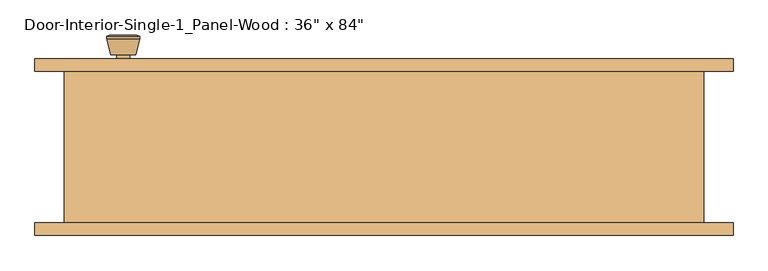
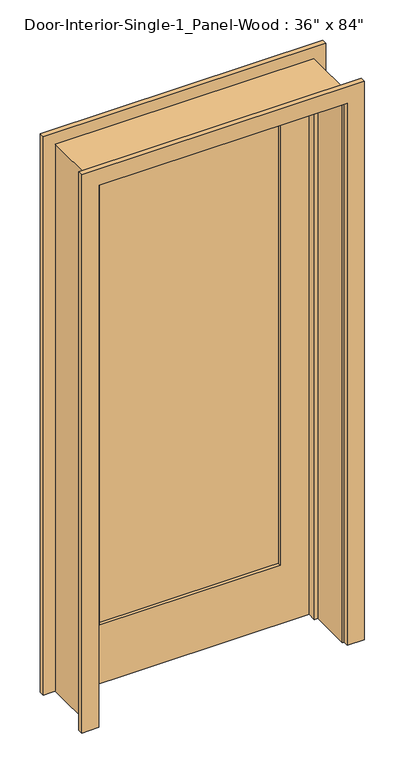
"""IFC4 building model written with IfcOpenShell, lengths in millimetres: door geometry."""

from ifc_helpers import new_model, si_unit, point, frame, frame_2d, origin, place, context, project, spatial, polyline, circle_curve, trimmed, segment, composite_curve, outline, extrude, faceted_brep, source, transform, mapped, element, save
from ifc_brep_helpers import plane_surface, cylinder_surface, revolved_surface, advanced_brep


def door_3b97b8e7(model_context):
    return source(origin(), model_context, "Body", "SolidModel", [
        advanced_brep(
        [(-393.7, 70.2, 914.4), (-383.7, 70.2, 914.4), (-403.7, 70.2, 914.4), (-373.2241324, 21.2, 914.4), (-393.7, 21.2, 914.4), (-414.1758676, 21.2, 914.4), (-368.7, 23.0278681, 914.4), (-418.7, 23.0278681, 914.4), (-368.7, 26.4915463, 914.4), (-418.7, 26.4915463, 914.4), (-375.063764, 51.2, 914.4), (-412.336236, 51.2, 914.4), (-383.7, 51.2, 914.4), (-403.7, 51.2, 914.4)],
        [
            (0, 1),
            (1, 2, circle_curve(frame((-393.7, 70.2, 914.4), z_axis=(0.0, 1.0, 0.0), x_axis=(-1.0, 0.0, 0.0)), 10.0)),
            (2, 0),
            (2, 1, circle_curve(frame((-393.7, 70.2, 914.4), z_axis=(0.0, 1.0, 0.0), x_axis=(-1.0, 0.0, 0.0)), 10.0)),
            (3, 4),
            (4, 5),
            (5, 3, circle_curve(frame((-393.7, 21.2, 914.4), z_axis=(0.0, -1.0, 0.0), x_axis=(-1.0, 0.0, 0.0)), 20.4758676)),
            (3, 5, circle_curve(frame((-393.7, 21.2, 914.4), z_axis=(0.0, -1.0, 0.0), x_axis=(-1.0, 0.0, 0.0)), 20.4758676)),
            (6, 3),
            (5, 7),
            (7, 6, circle_curve(frame((-393.7, 23.0278681, 914.4), z_axis=(0.0, -1.0, 0.0), x_axis=(-1.0, 0.0, 0.0)), 25.0)),
            (6, 7, circle_curve(frame((-393.7, 23.0278681, 914.4), z_axis=(0.0, -1.0, 0.0), x_axis=(-1.0, 0.0, 0.0)), 25.0)),
            (8, 6),
            (7, 9),
            (9, 8, circle_curve(frame((-393.7, 26.4915463, 914.4), z_axis=(0.0, -1.0, 0.0), x_axis=(-1.0, 0.0, 0.0)), 25.0)),
            (8, 9, circle_curve(frame((-393.7, 26.4915463, 914.4), z_axis=(0.0, -1.0, 0.0), x_axis=(-1.0, 0.0, 0.0)), 25.0)),
            (10, 8),
            (9, 11),
            (11, 10, circle_curve(frame((-393.7, 51.2, 914.4), z_axis=(0.0, -1.0, 0.0), x_axis=(-1.0, 0.0, 0.0)), 18.636236)),
            (10, 11, circle_curve(frame((-393.7, 51.2, 914.4), z_axis=(0.0, -1.0, 0.0), x_axis=(-1.0, 0.0, 0.0)), 18.636236)),
            (12, 10),
            (11, 13),
            (13, 12, circle_curve(frame((-393.7, 51.2, 914.4), z_axis=(0.0, -1.0, 0.0), x_axis=(-1.0, 0.0, 0.0)), 10.0)),
            (12, 13, circle_curve(frame((-393.7, 51.2, 914.4), z_axis=(0.0, -1.0, 0.0), x_axis=(-1.0, 0.0, 0.0)), 10.0)),
            (1, 12),
            (13, 2),
        ],
        [
            plane_surface(frame((-393.7, 70.2, 914.4), z_axis=(0.0, 1.0, 0.0), x_axis=(-1.0, 0.0, 0.0))),
            plane_surface(frame((-393.7, 21.2, 914.4), z_axis=(0.0, -1.0, 0.0), x_axis=(-1.0, 0.0, 0.0))),
            revolved_surface(polyline([(-414.1758676, 21.2, 914.4), (-418.7, 23.0278681, 914.4)]), (-393.7, 70.2, 914.4), (0.0, 1.0, 0.0)),
            cylinder_surface(frame((-393.7, 70.2, 914.4), z_axis=(0.0, 1.0, 0.0), x_axis=(-1.0, 0.0, 0.0)), 25.0),
            revolved_surface(polyline([(-418.7, 26.4915463, 914.4), (-412.336236, 51.2, 914.4)]), (-393.7, 70.2, 914.4), (0.0, 1.0, 0.0)),
            plane_surface(frame((-393.7, 51.2, 914.4), z_axis=(0.0, 1.0, 0.0), x_axis=(-1.0, 0.0, 0.0))),
            cylinder_surface(frame((-393.7, 70.2, 914.4), z_axis=(0.0, 1.0, 0.0), x_axis=(-1.0, 0.0, 0.0)), 10.0),
        ],
        [
            (0, [[1, 2, 3]]),
            (0, [[-3, 4, -1]]),
            (1, [[5, 6, 7]]),
            (1, [[-6, -5, 8]]),
            (2, [[9, -7, 10, 11]]),
            (2, [[-10, -8, -9, 12]]),
            (3, [[13, -11, 14, 15]]),
            (3, [[-14, -12, -13, 16]]),
            (4, [[17, -15, 18, 19]]),
            (4, [[-18, -16, -17, 20]]),
            (5, [[21, -19, 22, 23]]),
            (5, [[-22, -20, -21, 24]]),
            (6, [[25, -23, 26, -2]]),
            (6, [[-26, -24, -25, -4]]),
        ],
    ),
        extrude(outline(composite_curve([segment(trimmed(circle_curve(frame_2d((914.4, -393.7)), 30.0), [point((914.4, -423.7))], [point((914.4, -363.7))], False, "CARTESIAN"), True, "CONTINUOUS"), segment(trimmed(circle_curve(frame_2d((914.4, -393.7)), 30.0), [point((914.4, -363.7))], [point((914.4, -423.7))], False, "CARTESIAN"), True, "CONTINUOUS")], self_intersect=False)), frame((0.0, 70.2, 0.0), z_axis=(0.0, 1.0, 0.0), x_axis=(0.0, 0.0, 1.0)), (0.0, 0.0, 1.0), 6.0),
        advanced_brep(
        [(-393.7, 117.125, 914.4), (-403.7, 117.125, 914.4), (-383.7, 117.125, 914.4), (-373.2241324, 166.125, 914.4), (-414.1758676, 166.125, 914.4), (-393.7, 166.125, 914.4), (-368.7, 164.2971319, 914.4), (-418.7, 164.2971319, 914.4), (-368.7, 160.8334537, 914.4), (-418.7, 160.8334537, 914.4), (-375.063764, 136.125, 914.4), (-412.336236, 136.125, 914.4), (-383.7, 136.125, 914.4), (-403.7, 136.125, 914.4)],
        [
            (0, 1),
            (1, 2, circle_curve(frame((-393.7, 117.125, 914.4), z_axis=(0.0, -1.0, 0.0), x_axis=(-1.0, 0.0, 0.0)), 10.0)),
            (2, 0),
            (2, 1, circle_curve(frame((-393.7, 117.125, 914.4), z_axis=(0.0, -1.0, 0.0), x_axis=(-1.0, 0.0, 0.0)), 10.0)),
            (3, 4, circle_curve(frame((-393.7, 166.125, 914.4), z_axis=(0.0, 1.0, 0.0), x_axis=(-1.0, 0.0, 0.0)), 20.4758676)),
            (4, 5),
            (5, 3),
            (4, 3, circle_curve(frame((-393.7, 166.125, 914.4), z_axis=(0.0, 1.0, 0.0), x_axis=(-1.0, 0.0, 0.0)), 20.4758676)),
            (6, 7, circle_curve(frame((-393.7, 164.2971319, 914.4), z_axis=(0.0, 1.0, 0.0), x_axis=(-1.0, 0.0, 0.0)), 25.0)),
            (7, 4),
            (3, 6),
            (7, 6, circle_curve(frame((-393.7, 164.2971319, 914.4), z_axis=(0.0, 1.0, 0.0), x_axis=(-1.0, 0.0, 0.0)), 25.0)),
            (8, 9, circle_curve(frame((-393.7, 160.8334537, 914.4), z_axis=(0.0, 1.0, 0.0), x_axis=(-1.0, 0.0, 0.0)), 25.0)),
            (9, 7),
            (6, 8),
            (9, 8, circle_curve(frame((-393.7, 160.8334537, 914.4), z_axis=(0.0, 1.0, 0.0), x_axis=(-1.0, 0.0, 0.0)), 25.0)),
            (10, 11, circle_curve(frame((-393.7, 136.125, 914.4), z_axis=(0.0, 1.0, 0.0), x_axis=(-1.0, 0.0, 0.0)), 18.636236)),
            (11, 9),
            (8, 10),
            (11, 10, circle_curve(frame((-393.7, 136.125, 914.4), z_axis=(0.0, 1.0, 0.0), x_axis=(-1.0, 0.0, 0.0)), 18.636236)),
            (12, 13, circle_curve(frame((-393.7, 136.125, 914.4), z_axis=(0.0, 1.0, 0.0), x_axis=(-1.0, 0.0, 0.0)), 10.0)),
            (13, 11),
            (10, 12),
            (13, 12, circle_curve(frame((-393.7, 136.125, 914.4), z_axis=(0.0, 1.0, 0.0), x_axis=(-1.0, 0.0, 0.0)), 10.0)),
            (1, 13),
            (12, 2),
        ],
        [
            plane_surface(frame((-393.7, 117.125, 914.4), z_axis=(0.0, -1.0, 0.0), x_axis=(-1.0, 0.0, 0.0))),
            plane_surface(frame((-393.7, 166.125, 914.4), z_axis=(0.0, 1.0, 0.0), x_axis=(-1.0, 0.0, 0.0))),
            revolved_surface(polyline([(-414.1758676, 166.125, 914.4), (-418.7, 164.2971319, 914.4)]), (-393.7, 117.125, 914.4), (0.0, -1.0, 0.0)),
            cylinder_surface(frame((-393.7, 117.125, 914.4), z_axis=(0.0, -1.0, 0.0), x_axis=(-1.0, 0.0, 0.0)), 25.0),
            revolved_surface(polyline([(-418.7, 160.8334537, 914.4), (-412.336236, 136.125, 914.4)]), (-393.7, 117.125, 914.4), (0.0, -1.0, 0.0)),
            plane_surface(frame((-393.7, 136.125, 914.4), z_axis=(0.0, -1.0, 0.0), x_axis=(-1.0, 0.0, 0.0))),
            cylinder_surface(frame((-393.7, 117.125, 914.4), z_axis=(0.0, -1.0, 0.0), x_axis=(-1.0, 0.0, 0.0)), 10.0),
        ],
        [
            (0, [[1, 2, 3]]),
            (0, [[-3, 4, -1]]),
            (1, [[5, 6, 7]]),
            (1, [[8, -7, -6]]),
            (2, [[9, 10, -5, 11]]),
            (2, [[12, -11, -8, -10]]),
            (3, [[13, 14, -9, 15]]),
            (3, [[16, -15, -12, -14]]),
            (4, [[17, 18, -13, 19]]),
            (4, [[20, -19, -16, -18]]),
            (5, [[21, 22, -17, 23]]),
            (5, [[24, -23, -20, -22]]),
            (6, [[-2, 25, -21, 26]]),
            (6, [[-4, -26, -24, -25]]),
        ],
    ),
        extrude(outline(composite_curve([segment(trimmed(circle_curve(frame_2d((914.4, -393.7)), 30.0), [point((914.4, -423.7))], [point((914.4, -363.7))], False, "CARTESIAN"), True, "CONTINUOUS"), segment(trimmed(circle_curve(frame_2d((914.4, -393.7)), 30.0), [point((914.4, -363.7))], [point((914.4, -423.7))], False, "CARTESIAN"), True, "CONTINUOUS")], self_intersect=False)), frame((0.0, 111.125, 0.0), z_axis=(0.0, 1.0, 0.0), x_axis=(0.0, 0.0, 1.0)), (0.0, 0.0, 1.0), 6.0),
        faceted_brep([(482.6, 111.125, 0.0), (482.6, -117.475, 0.0), (457.2, -117.475, 0.0), (457.2, 41.275, 0.0), (444.5, 41.275, 0.0), (444.5, 76.2, 0.0), (457.2, 76.2, 0.0), (457.2, 111.125, 0.0), (482.6, 111.125, 2159.0), (482.6, -117.475, 2159.0), (-482.6, -117.475, 2159.0), (-482.6, -117.475, 0.0), (-457.2, -117.475, 0.0), (-457.2, -117.475, 2133.6), (457.2, -117.475, 2133.6), (457.2, 41.275, 2133.6), (-457.2, 41.275, 2133.6), (-457.2, 41.275, 0.0), (-444.5, 41.275, 0.0), (-444.5, 41.275, 2120.9), (444.5, 41.275, 2120.9), (444.5, 76.2, 2120.9), (-444.5, 76.2, 2120.9), (-444.5, 76.2, 0.0), (-457.2, 76.2, 0.0), (-457.2, 76.2, 2133.6), (457.2, 76.2, 2133.6), (457.2, 111.125, 2133.6), (-457.2, 111.125, 2133.6), (-457.2, 111.125, 0.0), (-482.6, 111.125, 0.0), (-482.6, 111.125, 2159.0)], [[[0, 1, 2, 3, 4, 5, 6, 7]], [[1, 0, 8, 9]], [[2, 1, 9, 10, 11, 12, 13, 14]], [[3, 2, 14, 15]], [[4, 3, 15, 16, 17, 18, 19, 20]], [[5, 4, 20, 21]], [[6, 5, 21, 22, 23, 24, 25, 26]], [[7, 6, 26, 27]], [[0, 7, 27, 28, 29, 30, 31, 8]], [[9, 8, 31, 10]], [[15, 14, 13, 16]], [[21, 20, 19, 22]], [[27, 26, 25, 28]], [[30, 29, 24, 23, 18, 17, 12, 11]], [[10, 31, 30, 11]], [[16, 13, 12, 17]], [[22, 19, 18, 23]], [[28, 25, 24, 29]]]),
        extrude(outline(polyline([(2133.6, -457.2), (0.0, -457.2), (0.0, 457.2), (2133.6, 457.2), (2133.6, -457.2)]), holes=[polyline([(2014.5375, -336.55), (2014.5375, 336.55), (231.775, 336.55), (231.775, -336.55), (2014.5375, -336.55)])]), frame((0.0, 76.2, 0.0), z_axis=(0.0, 1.0, 0.0), x_axis=(0.0, 0.0, 1.0)), (0.0, 0.0, 1.0), 34.925),
        extrude(outline(polyline([(336.55, 87.8416667), (-336.55, 87.8416667), (-336.55, 99.4833333), (336.55, 99.4833333), (336.55, 87.8416667)])), frame((0.0, 0.0, 231.775), z_axis=(0.0, 0.0, 1.0), x_axis=(1.0, 0.0, 0.0)), (0.0, 0.0, 1.0), 1782.7625),
        extrude(outline(polyline([(0.0, 463.55), (0.0, 527.05), (2203.45, 527.05), (2203.45, -527.05), (0.0, -527.05), (0.0, -463.55), (2139.95, -463.55), (2139.95, 463.55), (0.0, 463.55)])), frame((0.0, 111.125, 0.0), z_axis=(0.0, 1.0, 0.0), x_axis=(0.0, 0.0, 1.0)), (0.0, 0.0, 1.0), 19.05),
        extrude(outline(polyline([(0.0, 463.55), (0.0, 527.05), (2203.45, 527.05), (2203.45, -527.05), (0.0, -527.05), (0.0, -463.55), (2139.95, -463.55), (2139.95, 463.55), (0.0, 463.55)])), frame((0.0, -136.525, 0.0), z_axis=(0.0, 1.0, 0.0), x_axis=(0.0, 0.0, 1.0)), (0.0, 0.0, 1.0), 19.05),
    ])


if __name__ == "__main__":
    model = new_model("IFC4")
    model_context = context("Model", 3, world=origin())
    ifc_project = project(units=[si_unit("LENGTHUNIT", "METRE", prefix="MILLI")], contexts=[model_context])
    site = spatial("IfcSite", under=ifc_project)
    building = spatial("IfcBuilding", under=site)
    placement = place(None, origin())
    door_shape = door_3b97b8e7(model_context)
    element("IfcDoor", 1, ObjectType="Door-Interior-Single-1_Panel-Wood : 36\" x 84\"", at=placement, inside=building, context=model_context, shape_type="MappedRepresentation", body=[
        mapped(door_shape, transform((0.0, 0.0, 0.0), x_axis=(1.0, 0.0, 0.0), y_axis=(0.0, 1.0, 0.0), z_axis=(0.0, 0.0, 1.0))),
    ])
    save(model, "model.ifc")

# Revit data of these elements
# Type "Door-Interior-Single-1_Panel-Wood : 36\" x 84\""
#   Type Mark = "8"
#   Assembly Code = "C1020300"
#   Analytic Construction = "Wooden"
#   Top Rail = 0' - 4 11/16"
#   Thickness = 0' - 1 3/8"
#   Thermal Resistance (R) = 2.5876 (h·ft²·°F)/BTU
#   Swing Angle [instance default] = 90.00°
#   Stiles = 0' - 4 3/4"
#   Rough Width = 3' - 2"
#   Rough Height = 7' - 1"
#   Height = 7' - 0"
#   Width = 3' - 0"
#   Heat Transfer Coefficient (U) = 0.3865 BTU/(h·ft²·°F)
#   Bottom Rail = 0' - 9 1/8"
#   Trim Material = Cherry
#   Panel Material = door
#   Frame Material = door
#   Door Handle Material = Aluminum
#   Visual Light Transmittance = 0
#   Solar Heat Gain Coefficient = 0
#   Wall Closure = (empty or 0)
#   Function = (empty or 0)
# Element 1 (IfcDoor, "Door-Interior-Single-1_Panel-Wood : 36\" x 84\"")
#   Materials on its faces: "Aluminum", "door", "Cherry"
# Materials
#   "Cherry": class "Wood", colour RGB 226 177 128, transparency 0, Description = "Prunus Serotina", Cost = 0
#   "door": class "Generic", colour RGB 120 120 120, transparency 0, Cost = 0
#   "Aluminum": class "Metal", colour RGB 247 247 247, transparency 0, Description = "Aluminum 6061", Cost = 0
